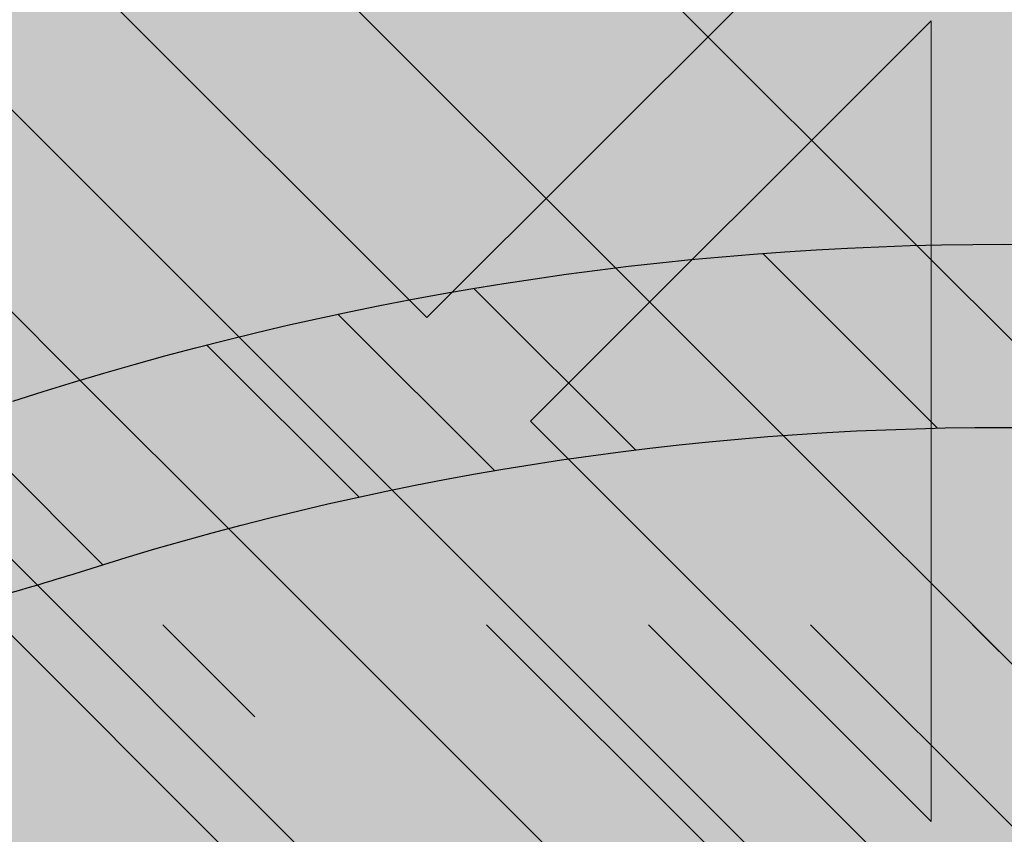
# Model space of a CAD drawing. Units: inches. Extents: x 844 to 2234, y 346 to 1084.
# Tile 80 of 93: x 2002.145 to 2003.858, y 707.323 to 708.742. Entities that reach past the tile are written whole.
import ezdxf

# ---------------------------------------------------------------- set-up
doc = ezdxf.new("R2010")
doc.units = ezdxf.units.IN
doc.header["$MEASUREMENT"] = 0
for name, color, linetype, lineweight in [('A-ANNO-DIMS', 2, 'Continuous', 18), ('furniture', 8, 'Continuous', 18), ('RA-AP-01$0$INT', 35, 'Continuous', 5)]:
    doc.layers.add(name, color=color, linetype=linetype, lineweight=lineweight)
doc.layers.add('RA-AP-01$0$FURN', color=3, linetype='Continuous')
doc.layers.add('RA-AP-01$0$WOOD', color=64, linetype='Continuous')
doc.styles.get("Standard").update_dxf_attribs({"font": 'arial.ttf'})
doc.dimstyles.get("Standard").update_dxf_attribs({"dimtxt": 6, "dimasz": 3, "dimexe": 0.18, "dimexo": 0.0625, "dimgap": 0.09, "dimtad": 0, "dimtih": 1, "dimtoh": 1, "dimdec": 1, "dimzin": 0, "dimdsep": 46, "dimlunit": 3, "dimtxsty": 'Standard', "dimblk": 'ARCHTICK', "dimcen": 0.09, "dimadec": 0, "dimazin": 0, "dimtfac": 1, "dimtdec": 1, "dimtofl": 0, "dimtmove": 0, "dimatfit": 3, "dimfxl": 1, "dimtolj": 1, "dimtzin": 0, "dimarcsym": 0})

# ---------------------------------------------------------------- blocks, each defined once
blk = doc.blocks.new('A$C18D01794')
at = {"layer": 'RA-AP-01$0$INT'}
h = blk.add_hatch(color=256, dxfattribs=at)
h.paths.add_polyline_path([(4.585917135068448, -7.856712009587804), (4.614201406330596, -7.856712009587056), (4.668846067270487, -7.802067348644738), (4.723490728212344, -7.856712009584164), (4.771774999457151, -7.856712009582887), (4.826419660396886, -7.80206734864072), (4.862780050090322, -7.838427738332541), (4.844495778842715, -7.856712009580965), (4.862780050090411, -7.856712009580482), (4.905206456960182, -7.814285602707865), (4.947632863832445, -7.856712009578238), (4.965917135079675, -7.856712009577755), (4.947632863831759, -7.838427738330656), (4.983993253523576, -7.802067348637219), (5.038637914464627, -7.856712009575829), (5.08692218571208, -7.856712009574554), (5.141566846649976, -7.802067348634224), (5.196211507589851, -7.856712009571666), (5.224495778822615, -7.856712009570916), (4.905206456953975, -7.537422687702283)])
h.paths.add_polyline_path([(4.895206456956031, -7.575706958950402), (4.895206456958921, -7.684996280828174), (4.840561796018589, -7.630351619890275)], flags=16)
h.paths.add_polyline_path([(4.915206456955638, -7.575706958949956), (4.969851117895509, -7.630351619887399), (4.915206456957609, -7.684996280827732)], flags=16)
h.paths.add_polyline_path([(4.826419660395175, -7.644493755514321), (4.881064321335613, -7.699138416452331), (4.771774999456703, -7.69913841645522)], flags=16)
h.paths.add_polyline_path([(4.983993253519558, -7.644493755510815), (5.038637914460456, -7.699138416449285), (4.929348592581548, -7.69913841645126)], flags=16)
h.paths.add_polyline_path([(4.881064321336025, -7.719138416452334), (4.826419660397532, -7.773783077393256), (4.771774999457062, -7.719138416455217)], flags=16)
h.paths.add_polyline_path([(4.929348592582019, -7.71913841645126), (5.038637914460982, -7.719138416449284), (4.983993253522945, -7.773783077389749)], flags=16)
h.paths.add_polyline_path([(4.895206456960191, -7.733280552075633), (4.895206456962115, -7.806001331460164), (4.876922185715016, -7.824285602708492), (4.840561796021581, -7.787925213016675)], flags=16)
h.paths.add_polyline_path([(4.915206456958487, -7.733280552075187), (4.969851117899527, -7.787925213013798), (4.933490728206909, -7.824285602708034), (4.9152064569598, -7.806001331461736)], flags=16)
h.paths.add_polyline_path([(4.757632863832376, -7.733280552079264), (4.812277524772842, -7.787925213017304), (4.757632863834348, -7.842569873958233)], flags=16)
h.paths.add_polyline_path([(4.737632863832376, -7.73328055207979), (4.737632863834348, -7.842569873958701), (4.682988202893906, -7.787925213020692)], flags=16)
h.paths.add_polyline_path([(5.05278005008503, -7.733280552072701), (5.052780050087917, -7.842569873951664), (4.998135389146995, -7.787925213013169)], flags=16)
h.paths.add_polyline_path([(5.072780050085024, -7.733280552072333), (5.127424711025931, -7.787925213010806), (5.072780050087916, -7.842569873951244)], flags=16)
h.paths.add_polyline_path([(4.935917135072783, -7.506712009583784), (5.255206456948811, -7.826001331459767), (5.255206456948932, -7.797717060211899), (5.200561796010279, -7.743072399273238), (5.255206456949403, -7.688427738334128), (5.25520645694961, -7.640143467086677), (5.200561796009787, -7.585498806146837), (5.236922185702417, -7.549138416454212), (5.255206456949919, -7.56742268770172), (5.255206456949998, -7.549138416454178), (5.212780050078687, -7.506712009583814), (5.25520645695036, -7.464285602712145), (5.255206456950438, -7.446001331464763), (5.236922185702424, -7.464285602712779), (5.200561796009796, -7.427925213020149), (5.255206456950753, -7.373280552079203), (5.25520645695096, -7.324996280834394), (5.200561796010322, -7.270351619893748), (5.255206456951428, -7.215706958952649), (5.255206456951547, -7.187422687705071)])
h.paths.add_polyline_path([(5.042988202883395, -7.42792521302065), (5.097632863823085, -7.373280552080975), (5.097632863822622, -7.482569873959883)], flags=16)
h.paths.add_polyline_path([(5.028846067259663, -7.442067348644384), (5.083490728198774, -7.496712009583504), (4.974201406321001, -7.496712009583035)], flags=16)
h.paths.add_polyline_path([(5.117632863823087, -7.37328055208089), (5.172277524762331, -7.42792521302015), (5.11763286382262, -7.482569873959851)], flags=16)
h.paths.add_polyline_path([(5.08349072819877, -7.516712009582191), (5.028846067259652, -7.571356670521302), (4.974201406320998, -7.516712009582638)], flags=16)
h.paths.add_polyline_path([(5.131774999446817, -7.35913841645716), (5.186419660386065, -7.413783077396415), (5.241064321325782, -7.359138416456712)], flags=17)
h.paths.add_polyline_path([(5.131774999446228, -7.496712009583703), (5.186419660386065, -7.442067348643883), (5.222780050079488, -7.478427738337313), (5.204495778832781, -7.496712009584014)], flags=16)
h.paths.add_polyline_path([(5.097632863822613, -7.530854145205813), (5.097632863823061, -7.640143467084723), (5.042988202883383, -7.585498806145032)], flags=16)
h.paths.add_polyline_path([(5.131774999446899, -7.339138416457162), (5.241064321325809, -7.339138416456712), (5.186419660386591, -7.284493755517479)], flags=17)
h.paths.add_polyline_path([(5.131774999446226, -7.516712009581999), (5.204495778830767, -7.516712009581702), (5.22278005007868, -7.534996280829206), (5.186419660386049, -7.571356670521828)], flags=16)
h.paths.add_polyline_path([(5.11763286382262, -7.530854145205852), (5.17227752476232, -7.585498806145562), (5.117632863823064, -7.64014346708481)], flags=16)
h.paths.add_polyline_path([(5.186419660386069, -7.599640941770585), (5.241064321325754, -7.654285602710281), (5.131774999446791, -7.654285602709814)], flags=16)
h.paths.add_polyline_path([(5.131774999446872, -7.674285602709813), (5.24106432132578, -7.674285602710282), (5.186419660386554, -7.728930263649504)], flags=16)
h.paths.add_polyline_path([(5.255206456951811, -7.126001331467467), (5.255206456951895, -7.106712009588038), (4.555206456956052, -7.106712009588038), (4.555206456956136, -7.12600133146746), (4.905206456953973, -7.476001331465289)])
h.paths.add_polyline_path([(4.983993253513404, -7.368930263651977), (4.92934859257295, -7.314285602713969), (5.03863791445186, -7.314285602711063)], flags=16)
h.paths.add_polyline_path([(4.969851117889988, -7.383072399276016), (4.915206456952556, -7.437717060215906), (4.915206456949648, -7.328427738338133)], flags=16)
h.paths.add_polyline_path([(4.929348592572535, -7.294285602713971), (4.983993253511019, -7.239640941773039), (5.038637914451496, -7.294285602711065)], flags=16)
h.paths.add_polyline_path([(5.052780050074912, -7.280143467087016), (4.998135389134438, -7.225498806148989), (5.052780050072919, -7.170854145208052)], flags=16)
h.paths.add_polyline_path([(5.07278005007491, -7.280143467086489), (5.072780050072918, -7.170854145207579), (5.127424711013374, -7.225498806145578)], flags=16)
h.paths.add_polyline_path([(4.89520645695295, -7.437717060216355), (4.840561796013067, -7.383072399278919), (4.895206456950961, -7.328427738338582)], flags=16)
h.paths.add_polyline_path([(4.915206456948365, -7.280143467090674), (4.915206456946434, -7.207422687704125), (4.933490728192729, -7.18913841645701), (4.969851117886972, -7.225498806149623)], flags=16)
h.paths.add_polyline_path([(4.881064321327021, -7.314285602715054), (4.82641966038902, -7.368930263655506), (4.771774999448108, -7.314285602717047)], flags=16)
h.paths.add_polyline_path([(4.895206456950073, -7.280143467091125), (4.840561796009022, -7.225498806152518), (4.876922185700835, -7.18913841645908), (4.895206456948749, -7.207422687706589)], flags=16)
h.paths.add_polyline_path([(4.983993253510392, -7.211356670525576), (4.947632863816944, -7.174996280833758), (4.965917135064043, -7.156712009585847), (5.038637914448995, -7.156712009584522)], flags=16)
h.paths.add_polyline_path([(4.881064321326543, -7.294285602715056), (4.771774999447578, -7.294285602717046), (4.826419660385607, -7.239640941776569)], flags=16)
h.paths.add_polyline_path([(4.905206456946447, -7.19913841645844), (4.862780050074785, -7.156712009587725), (4.947632863816685, -7.156712009586302)], flags=16)
h.paths.add_polyline_path([(5.14156684663679, -7.211356670521528), (5.086922185696452, -7.156712009583639), (5.196211507574223, -7.156712009581651)], flags=16)
h.paths.add_polyline_path([(4.8264196603837, -7.211356670529104), (4.771774999442643, -7.156712009590501), (4.8444957788276, -7.156712009588568), (4.862780050075511, -7.17499628083566)], flags=16)
h.paths.add_polyline_path([(4.812277524760289, -7.225498806153156), (4.757632863822258, -7.28014346709363), (4.757632863819352, -7.170854145214669)], flags=16)
h.paths.add_polyline_path([(4.73763286382226, -7.280143467093997), (4.682988202881349, -7.22549880615554), (4.737632863819352, -7.170854145215086)], flags=16)
h.paths.add_polyline_path([(4.723490728195188, -7.156712009591787), (4.668846067257299, -7.211356670532127), (4.614201406317417, -7.156712009594693)], flags=16)
h.paths.add_polyline_path([(4.597632863829262, -7.506712009583814), (4.555206456957951, -7.54913841645418), (4.555206456958029, -7.56742268770172), (4.573490728205535, -7.549138416454212), (4.609851117898167, -7.585498806146839), (4.555206456958338, -7.640143467086675), (4.555206456958546, -7.688427738334125), (4.60985111789767, -7.743072399273238), (4.555206456959015, -7.797717060211899), (4.555206456959138, -7.826001331459767), (4.874495778835167, -7.506712009583786), (4.5552064569564, -7.187422687705062), (4.555206456956523, -7.215706958952644), (4.609851117897629, -7.270351619893746), (4.555206456956988, -7.324996280834396), (4.555206456957198, -7.373280552079195), (4.609851117898153, -7.427925213020147), (4.573490728205528, -7.464285602712779), (4.555206456957507, -7.446001331464756), (4.555206456957585, -7.464285602712143)])
h.paths.add_polyline_path([(4.712780050085332, -7.482569873959882), (4.712780050084863, -7.373280552080972), (4.767424711024555, -7.42792521302065)], flags=16)
h.paths.add_polyline_path([(4.726922185709173, -7.496712009583504), (4.781566846648288, -7.442067348644384), (4.836211507586949, -7.496712009583033)], flags=16)
h.paths.add_polyline_path([(4.692780050085327, -7.482569873959851), (4.638135389145619, -7.427925213020149), (4.692780050084865, -7.373280552080892)], flags=16)
h.paths.add_polyline_path([(4.726922185709182, -7.516712009582191), (4.836211507586949, -7.51671200958264), (4.7815668466483, -7.571356670521304)], flags=16)
h.paths.add_polyline_path([(4.678637914461726, -7.496712009583706), (4.605917135075169, -7.496712009584014), (4.587632863828464, -7.478427738337311), (4.623993253521887, -7.442067348643881)], flags=16)
h.paths.add_polyline_path([(4.712780050085336, -7.530854145205816), (4.767424711024568, -7.585498806145034), (4.71278005008489, -7.640143467084724)], flags=16)
h.paths.add_polyline_path([(4.678637914461726, -7.516712009582001), (4.623993253521899, -7.571356670521829), (4.587632863829271, -7.534996280829206), (4.605917135077185, -7.5167120095817)], flags=16)
h.paths.add_polyline_path([(4.692780050085336, -7.530854145205848), (4.692780050084889, -7.64014346708481), (4.638135389145632, -7.585498806145562)], flags=16)
h.paths.add_polyline_path([(4.623993253521885, -7.413783077396415), (4.678637914461131, -7.359138416457161), (4.56934859258217, -7.359138416456712)], flags=17)
h.paths.add_polyline_path([(4.623993253521901, -7.599640941770568), (4.678637914461158, -7.654285602709814), (4.569348592582195, -7.654285602710281)], flags=16)
h.paths.add_polyline_path([(4.678637914461051, -7.339138416457162), (4.623993253521361, -7.284493755517479), (4.569348592582143, -7.339138416456712)], flags=17)
h.paths.add_polyline_path([(4.678637914461076, -7.674285602709813), (4.623993253521399, -7.728930263649504), (4.569348592582167, -7.674285602710281)], flags=16)
h = blk.add_hatch(color=256, dxfattribs=at)
h.paths.add_polyline_path([(4.905206456954232, -7.537422687702028), (4.874495778835232, -7.506712009583718), (4.555206456959138, -7.826001331459766), (4.555206456959269, -7.856712009588616), (4.585917135068449, -7.856712009587804)])
h.paths.add_polyline_path([(4.935917135072152, -7.506712009583152), (4.905206456953497, -7.537422687701806), (5.224495778822614, -7.856712009570917), (5.255206456948681, -7.856712009570104), (5.255206456948813, -7.826001331459768)])
h.paths.add_polyline_path([(5.255206456951549, -7.18742268770507), (5.255206456951813, -7.126001331467461), (4.905206456953563, -7.476001331465701), (4.935917135072559, -7.506712009584006)])
h.paths.add_polyline_path([(4.874495778835167, -7.506712009583785), (4.905206456953818, -7.476001331465132), (4.555206456956135, -7.126001331467458), (4.555206456956399, -7.187422687705064)])
h = blk.add_hatch(color=256, dxfattribs=at)
h.paths.add_polyline_path([(4.969851117891331, -7.630351619889621), (4.915206456952669, -7.575706958950966), (4.915206456952222, -7.684996280828739)])
h.paths.add_polyline_path([(4.895206456953064, -7.575706958950968), (4.840561796014413, -7.630351619889628), (4.895206456953533, -7.684996280828741)])
h.paths.add_polyline_path([(4.826419660390684, -7.644493755513362), (4.771774999451003, -7.699138416453052), (4.881064321329913, -7.699138416452587)])
h.paths.add_polyline_path([(4.881064321329884, -7.719138416452585), (4.771774999450921, -7.719138416453052), (4.82641966039018, -7.773783077392298)])
h.paths.add_polyline_path([(4.895206456953734, -7.733280552076196), (4.840561796013912, -7.787925213016031), (4.876922185707337, -7.824285602709455), (4.895206456954043, -7.806001331462747)])
h.paths.add_polyline_path([(4.862780050082808, -7.838427738332388), (4.826419660390178, -7.802067348639763), (4.771774999450351, -7.856712009579595), (4.844495778835303, -7.856712009579895)])
h.paths.add_polyline_path([(4.812277524766446, -7.787925213016036), (4.757632863827191, -7.733280552076788), (4.757632863826741, -7.842569873955747)])
h.paths.add_polyline_path([(4.737632863827191, -7.733280552076863), (4.682988202887508, -7.787925213016558), (4.737632863826743, -7.842569873955778)])
h.paths.add_polyline_path([(4.668846067263777, -7.802067348640287), (4.614201406325123, -7.856712009578949), (4.723490728202894, -7.856712009579402)])
h.paths.add_polyline_path([(4.905206456953846, -7.814285602708654), (4.862780050082654, -7.856712009579847), (4.947632863824561, -7.85671200958032)])
h.paths.add_polyline_path([(4.915206456952028, -7.733280552076195), (4.91520645695173, -7.806001331460731), (4.933490728199234, -7.824285602708648), (4.96985111789186, -7.787925213016022)])
h.paths.add_polyline_path([(5.038637914454841, -7.719138416453029), (4.929348592575874, -7.71913841645258), (4.983993253515593, -7.773783077392289)])
h.paths.add_polyline_path([(4.983993253515065, -7.644493755513352), (4.929348592575849, -7.699138416452582), (5.038637914454755, -7.699138416453031)])
h.paths.add_polyline_path([(5.052780050079843, -7.73328055207676), (4.998135389140595, -7.787925213016018), (5.052780050080309, -7.842569873955721)])
h.paths.add_polyline_path([(4.983993253516868, -7.802067348639752), (4.947632863824241, -7.838427738332383), (4.965917135071747, -7.856712009579888), (5.038637914456701, -7.856712009579572)])
h.paths.add_polyline_path([(5.127424711019533, -7.787925213016519), (5.072780050079843, -7.733280552076838), (5.07278005008031, -7.842569873955751)])
h.paths.add_polyline_path([(5.141566846643269, -7.802067348640248), (5.086922185704154, -7.85671200957937), (5.196211507581929, -7.856712009578901)])
for p, q in [((4.935917135072783, -7.506712009583784), (5.255206456948813, -7.826001331459769)), ((4.905206456953975, -7.537422687702283), (5.224495778822613, -7.856712009570916)), ((4.915206456955636, -7.575706958949957), (4.969851117895507, -7.630351619887399)), ((4.915206456957609, -7.684996280827729), (4.915206456955636, -7.575706958949957)), ((4.915206456957613, -7.684996280827727), (4.969851117895507, -7.630351619887399)), ((4.929348592581546, -7.69913841645126), (4.983993253519556, -7.644493755510815)), ((4.983993253519558, -7.644493755510817), (5.038637914460456, -7.699138416449285))]:
    blk.add_line(p, q, dxfattribs=at)
blk = doc.blocks.new('A$C32926AE1')
at = {"layer": 'RA-AP-01$0$FURN'}
h = blk.add_hatch(dxfattribs=at)
h.set_pattern_fill('ANSI31', color=256, scale=0.1, style=0)
h.set_pattern_definition([(45, (0, 0), (-0.0088388347648318, 0.0088388347648318), [])])
edge = h.paths.add_edge_path(flags=16)
edge.add_arc((4.904771284329206, 4.246793130718756), 0.2603971832811541, 75.22398030683196, 104.7760196931204)
edge.add_arc((4.904771284329206, 4.246793130718756), 0.2603971832811541, 75.223980306832, 104.77601969312039, ccw=False)
edge = h.paths.add_edge_path(flags=16)
edge.add_arc((4.904771284329206, 4.067062675376612), 0.2603971832811541, 255.2239803068796, 284.776019693168)
edge.add_arc((4.904771284329206, 4.067062675376612), 0.2603971832811541, 255.22398030687958, 284.77601969316805, ccw=False)
edge = h.paths.add_edge_path(flags=0)
edge.add_arc((4.904771284329206, 4.067062675376612), 0.2603971832811541, 255.2239803068796, 284.776019693168)
edge.add_arc((4.904771284329206, 4.067062675376612), 0.2603971832811541, 255.22398030687958, 284.77601969316805, ccw=False)
edge = h.paths.add_edge_path(flags=0)
edge.add_arc((4.904771284329206, 4.067062675376612), 0.2603971832811541, 255.2239803068796, 284.776019693168)
edge.add_arc((4.904771284329206, 4.067062675376612), 0.2603971832811541, 255.22398030687958, 284.77601969316805, ccw=False)
edge = h.paths.add_edge_path()
edge.add_arc((4.604388392048174, 4.588829985554312), 0.1599999999999918, 342.3781640246255, 354.4317409793762)
edge.add_arc((5.090145208887507, 4.43216705527679), 0.3503971832811637, 162.0091218307731, 180.3186872093483)
edge.add_arc((5.205154176610243, 4.588829985554953), 0.1599999999999917, 185.5682590208461, 197.6218359767349)
edge.add_arc((4.904771284329229, 4.246793130718735), 0.3503971832811761, 72.00912183053516, 107.9908781690354)
edge.add_arc((9.535952835716557, 4.28682295566602), 4.798342501046485, 178.2875002453811, 181.5576802719453)
edge.add_arc((4.719397359771122, 4.43216705527679), 0.3503971832811637, 359.6813127906516, 377.9908781692269)
edge.add_arc((9.535967292294904, 4.286822350292874), 4.778371420254705, 178.2965938931842, 181.5667745797229)
edge.add_arc((4.719397359771122, 4.43216705527679), 0.3303971832811637, 359.6813127906516, 377.9908781692269)
edge.add_arc((0.2735752763637294, 4.286822350292874), 4.7783714202547, 358.4332254202771, 361.7034061068158)
edge.add_arc((5.061434214606998, 4.732549947558029), 0.1600000000000254, 252.3781640250584, 264.4317409792362)
edge.add_arc((4.748108354051257, 4.732549947558012), 0.1600000000000541, 275.5682590208426, 287.6218359759532)
edge.add_arc((4.604388392048115, 4.588829985554317), 0.1800000000000505, 342.3567572500182, 349.3735009646207)
edge.add_arc((5.205154176610254, 4.588829985554976), 0.1800000000000069, 190.6264990356027, 197.6432427513933)
edge.add_arc((5.061434214607106, 4.732549947558013), 0.1800000000000424, 252.3567572496606, 259.3735009644582)
edge.add_arc((4.904771284329208, 4.246793130718737), 0.3303971832811676, 71.99844483668534, 108.0015551637021)
edge.add_arc((4.748108354051414, 4.732549947558045), 0.1800000000000547, 280.6264990355479, 287.6432427495938)
edge.add_arc((5.090145208887514, 4.432167055276789), 0.2803971832811691, 162.8706300666893, 180.816523289902)
edge.add_arc((4.719397359771136, 4.432167055276689), 0.2803971832811534, 359.183476710103, 377.1293699333214)
edge.add_arc((4.904771284329222, 4.246793130718737), 0.2803971832811769, 72.87063006672916, 107.1293699332334)
edge.add_arc((5.090145208887522, 4.432167055276788), 0.2603971832811776, 165.2239803068007, 180.9953123810312)
edge.add_arc((4.719397359771141, 4.432167055276699), 0.2603971832811458, 359.0046876189768, 374.7760196932087)
edge.add_arc((5.090145208887507, 4.43216705527679), 0.3303971832811637, 162.0091218307731, 180.3186872093483)
edge.add_arc((9.53595427642584, 4.285015535491528), 4.728345371032053, 178.265043920078, 181.5679956281801)
edge.add_arc((0.2735882922327999, 4.285015535491582), 4.728345371032045, 358.4320043718193, 361.7349560799204)
edge.add_arc((9.535953591267507, 4.284458026472751), 4.708343996644348, 178.2573054306777, 181.5704995759608)
edge.add_arc((0.273588977391114, 4.284458026472785), 4.708343996644358, 358.4295004240388, 361.7426945693213)
edge.add_arc((0.2735889773911131, 4.029397779622582), 4.708343996644359, 358.2573054306787, 361.5704995759613)
edge.add_arc((9.535953591267518, 4.029397779622618), 4.708343996644359, 178.4295004240391, 181.7426945693223)
edge.add_arc((0.2735882922327901, 4.028840270603786), 4.728345371032054, 358.2650439200796, 361.5679956281808)
edge.add_arc((9.53595427642584, 4.028840270603841), 4.728345371032054, 178.4320043718199, 181.7349560799219)
edge.add_arc((0.2735752763637302, 4.027033455802493), 4.778371420254699, 358.2965938931842, 361.5667745797229)
edge.add_arc((4.719397359771122, 3.881688750818578), 0.3303971832811637, 342.0091218307731, 360.3186872093484)
edge.add_arc((5.090145208887507, 3.881688750818578), 0.3303971832811637, 179.6813127906516, 197.9908781692269)
edge.add_arc((9.535967292294904, 4.027033455802493), 4.778371420254705, 178.433225420277, 181.7034061068158)
edge.add_arc((4.719397359771122, 3.881688750818578), 0.3503971832811637, 342.0091218307731, 360.3186872093484)
edge.add_arc((9.53595283571655, 4.027032850429349), 4.79834250104648, 178.4423197280546, 181.7124997546188)
edge.add_arc((4.719397359771141, 3.881688750818669), 0.2603971832811458, 345.2239803067913, 360.9953123810232)
edge.add_arc((5.090145208887522, 3.88168875081858), 0.2603971832811776, 179.0046876189687, 194.7760196931993)
edge.add_arc((4.904771284329222, 4.067062675376631), 0.2803971832811769, 252.8706300667665, 287.1293699332708)
edge.add_arc((4.719397359771136, 3.881688750818678), 0.2803971832811534, 342.8706300666787, 360.8165232898969)
edge.add_arc((5.090145208887514, 3.881688750818579), 0.2803971832811691, 179.183476710098, 197.1293699333106)
edge.add_arc((4.748108354051414, 3.581305858537323), 0.1800000000000547, 72.3567572504062, 79.37350096445199)
edge.add_arc((4.904771284329208, 4.067062675376631), 0.3303971832811676, 251.9984448362979, 288.0015551633146)
edge.add_arc((5.061434214607106, 3.581305858537355), 0.1800000000000424, 100.6264990355418, 107.6432427503394)
edge.add_arc((5.205154176610254, 3.725025820540392), 0.1800000000000069, 162.3567572486066, 169.3735009643972)
edge.add_arc((4.604388392048115, 3.725025820541051), 0.1800000000000505, 10.62649903537925, 17.64324274998182)
edge.add_arc((4.748108354051257, 3.581305858537356), 0.1600000000000541, 72.37816402404681, 84.43174097915735)
edge.add_arc((4.904771284329229, 4.067062675376632), 0.3503971832811761, 252.0091218309645, 287.9908781694648)
edge.add_arc((5.061434214606998, 3.581305858537339), 0.1600000000000254, 95.56825902076373, 107.6218359749416)
edge.add_arc((5.205154176610243, 3.725025820540414), 0.1599999999999917, 162.3781640232651, 174.4317409791539)
edge.add_arc((5.090145208887507, 3.881688750818578), 0.3503971832811637, 179.6813127906516, 197.9908781692269)
edge.add_arc((4.604388392048174, 3.725025820541056), 0.1599999999999918, 5.568259020623824, 17.62183597537444)
edge.add_arc((0.2735897329420762, 4.28682295566602), 4.798342501046482, 358.4423197280547, 361.7124997546188)
edge.add_arc((0.2735897329420691, 4.027032850429348), 4.798342501046489, 358.2875002453812, 361.5576802719453)
at = {"layer": 'RA-AP-01$0$WOOD'}
h = blk.add_hatch(color=256, dxfattribs=at)
h.dxf.hatch_style = 1
h.paths.add_polyline_path([(5.157430609644524, 4.573483066760929, -0.1009492694046607), (5.155401577623758, 4.593365984175333, -0.1842662638101597), (5.172249623284174, 4.638795604568598, 0.2056608120311276), (5.179560981299304, 4.661316324430096, 0.3614336704623542), (5.134352340494423, 4.706524965234944, 0.2056608120311297), (5.111831620632933, 4.699213607219793, -0.1842662638101113), (5.066402000239693, 4.682365561559342, -0.1055311479399994), (5.045656153913092, 4.68467289944697, 0.1567636581983829), (4.763886414745334, 4.684672899446966, -0.1055311479399895), (4.743140568418733, 4.68236556155934, -0.1842662638100833), (4.6977109480255, 4.69921360721979, 0.2056608120302612), (4.675190228164109, 4.706524965234949, 0.3614336704708441), (4.629981587358889, 4.66131632442871, 0.2056608120245944), (4.637292945374126, 4.638795604567974, -0.1842662638101024), (4.654140991034615, 4.59336598417475, -0.1009492694055169), (4.652111959013835, 4.573483066760181, 0.021410119221476), (4.629748025606143, 4.156712009541676, 0.0214101192214795), (4.652111959013809, 3.739940952323101, -0.1009492694059586), (4.654140991034615, 3.720058034908448, -0.1842662638100975), (4.637292945374126, 3.674628414515226, 0.2056608120245705), (4.629981587358889, 3.652107694654492, 0.3614336704708879), (4.675190228164113, 3.606899053848249, 0.2056608120302384), (4.697710948025501, 3.614210411863408, -0.1842662638100995), (4.743140568418738, 3.63105845752386, -0.1055311479402541), (4.763886414745388, 3.628751119636215, 0.1567636581983776), (5.045656153913137, 3.628751119636244, -0.1055311479397538), (5.066402000239692, 3.631058457523857, -0.1842662638101067), (5.111831620632931, 3.614210411863407, 0.2056608120310924), (5.134352340494417, 3.606899053848256, 0.3614336704624001), (5.179560981299307, 3.652107694653103, 0.2056608120311314), (5.172249623284175, 3.6746284145146, -0.1842662638101402), (5.155401577623758, 3.72005803490786, -0.1009492694051366), (5.15743060964455, 3.739940952322354, 0.0214101192215073), (5.179794543052287, 4.156712009541468, 0.0214101192215252)])
h.paths.add_polyline_path([(4.639748609479751, 4.156712009541513, 0.0213537860821624), (4.661970494867118, 3.741887061152232, -0.094075836301374), (4.664143710413708, 3.7196126951003, -0.1824818158568985), (4.644813765429836, 3.668037719127816, 0.2056608120245319), (4.639939526753007, 3.653023905887301, 0.3614336704710246), (4.676106439397173, 3.616856993242342, 0.2056608120302234), (4.691120252638095, 3.621731231919122, -0.1824818158602558), (4.742695228611606, 3.641061176902986, -0.1029891339458722), (4.766991894714349, 3.638256818950944, 0.156709409989566), (5.042550673941472, 3.638256818950105, -0.102989133958497), (5.066847340047078, 3.641061176902949, -0.1824818158594995), (5.118422316020358, 3.621731231919103, 0.2056608120311416), (5.133436129261316, 3.616856993242346, 0.3614336704621468), (5.169603041905217, 3.653023905886178, 0.2056608120310986), (5.164728803228477, 3.668037719127177, -0.1824818158565612), (5.145398858244737, 3.719612695099578, -0.0940758363009313), (5.147572073791232, 3.741887061151398, 0.0213537860822023), (5.169793959178681, 4.156712009541451, 0.0213537860822226), (5.147572073791203, 4.571536957931898, -0.0940758363005034), (5.145398858244737, 4.59381132398362, -0.1824818158565587), (5.164728803228476, 4.645386299956021, 0.2056608120311045), (5.169603041905216, 4.66040011319702, 0.3614336704621845), (5.133436129261313, 4.696567025840856, 0.2056608120310773), (5.118422316020359, 4.691692787164098, -0.182481815859508), (5.066847340047078, 4.67236284218025, -0.1029891339584606), (5.04255067394148, 4.675167200133092, 0.156709409989566), (4.766991894714357, 4.675167200132257, -0.1029891339458842), (4.742695228611611, 4.672362842180213, -0.1824818158602725), (4.691120252638095, 4.691692787164077, 0.2056608120302152), (4.676106439397174, 4.696567025840858, 0.3614336704710363), (4.639939526753005, 4.660400113195899, 0.2056608120245495), (4.644813765429837, 4.645386299955384, -0.1824818158568934), (4.664143710413708, 4.593811323982902, -0.0940758363009187), (4.661970494867149, 4.571536957931074, 0.021353786082177)], flags=16)
h.paths.add_polyline_path([(5.129794543052235, 4.432167055276933, -0.0141661062790638), (5.130152669293814, 4.156927903047693, -0.0141661062790647), (5.129794543052234, 3.881688750818433, -0.0785247771143638), (5.10979738006795, 3.755143611847103, 0.0945969212073497), (5.105408519571111, 3.717898134952927, 0.1043170707844957), (5.116074640131521, 3.670385395016088, 0.1043170707864965), (5.068561900193738, 3.681051515576561, 0.09459692119553), (5.031316423304057, 3.676662655080835, -0.1580239521427272), (4.778226145355827, 3.676662655080367, 0.0945969211986668), (4.740980668464973, 3.681051515576592, 0.1043170707882822), (4.693467928526415, 3.670385395015844, 0.1043170707867916), (4.704134049087309, 3.717898134953662, 0.0945969211972894), (4.69974518859162, 3.755143611844042, -0.0785247771163196), (4.679748025606343, 3.881688750818406, -0.0141661062790663), (4.679389899364763, 4.156927903047693, -0.0141661062790672), (4.679748025606343, 4.432167055276998, -0.0785247771163064), (4.699745188591625, 4.55871219425134, 0.094596921197333), (4.704134049087308, 4.595957671141738, 0.1043170707867205), (4.693467928526416, 4.643470411079523, 0.1043170707882628), (4.740980668464965, 4.632804290518776, 0.0945969211988114), (4.778226145355874, 4.637193151015016, -0.158023952142669), (5.031316423304015, 4.637193151014546, 0.0945969211956361), (5.068561900193736, 4.632804290518806, 0.1043170707864979), (5.11607464013152, 4.643470411079278, 0.1043170707844617), (5.105408519571112, 4.595957671142455, 0.0945969212074597), (5.109797380067959, 4.558712194248236, -0.0785247771143467)], flags=0)
h.paths.add_polyline_path([(5.119794532311105, 4.432259799204851, -0.0142000800617244), (5.120156169157484, 4.156927903047701, -0.0142000800617277), (5.119794532311105, 3.881596006890482, -0.0784894509520253), (5.100273383573699, 3.758192358677797, 0.0940138827242913), (5.095413455884425, 3.717477693979438, 0.0606271852308753), (5.099615656341024, 3.686844378806616, 0.0606271852322524), (5.068982341167493, 3.691046579263239, 0.0940138827010453), (5.028267676478798, 3.686186651576848, -0.1580706864508061), (4.781274892180912, 3.686186651576435, 0.0940138827026903), (4.740560227491556, 3.691046579263279, 0.0606271852339895), (4.709926912317155, 3.686844378806508, 0.0606271852329405), (4.714129112773991, 3.717477693980356, 0.094013882701304), (4.709269185087677, 3.758192358669163, -0.0784894509577193), (4.689748036347473, 3.881596006890469, -0.014200080061729), (4.689386399501094, 4.156927903047709, -0.0142000800617217), (4.689748036347473, 4.432259799204808, -0.078489450957724), (4.709269185087651, 4.555663447426125, 0.0940138827014585), (4.714129112773992, 4.596378112114996, 0.0606271852329731), (4.709926912317154, 4.62701142728886, 0.0606271852340196), (4.74056022749157, 4.622809226832087, 0.0940138827024997), (4.781274892180847, 4.627669154518912, -0.1580706864508359), (5.028267676478777, 4.627669154518526, 0.0940138827010946), (5.068982341167492, 4.622809226832129, 0.060627185232254), (5.099615656341024, 4.627011427288751, 0.0606271852308727), (5.095413455884425, 4.59637811211593, 0.0940138827241088), (5.100273383573675, 4.555663447417647, -0.0784894509520978)], flags=0)
h.paths.add_polyline_path([(5.06978912287499, 4.430218106756144, -0.014241683694547), (5.070173729147532, 4.156927903047672, -0.0142416836945458), (5.06978912287499, 3.883637699339223, -0.0800609523125196), (5.052662118612511, 3.773463122773442, 0.0526421978001116), (5.04590916754064, 3.740550867606997, 0.0526421977992423), (5.012996912374707, 3.73379791653534, -0.1583028414718258), (4.796545656286308, 3.73379791653451, 0.0526421978034211), (4.763633401117837, 3.740550867607021, 0.0526421978018622), (4.756880450045755, 3.773463122774558, -0.0800609523117106), (4.739753445783639, 3.883637699339268, -0.0142416836945435), (4.739368839511098, 4.156927903047671, -0.0142416836945477), (4.739753445783639, 4.430218106756155, -0.0800609523116345), (4.75688045004574, 4.540392683320762, 0.052642197801941), (4.763633401117837, 4.573304938488346, 0.0526421978035071), (4.796545656286361, 4.580057889560873, -0.1583028414717561), (5.012996912374669, 4.580057889560039, 0.0526421977993048), (5.04590916754064, 4.57330493848837, 0.0526421978002057), (5.052662118612529, 4.540392683321868, -0.080060952312477)], flags=0)
h.paths.add_polyline_path([(5.049789715110557, 4.43038092723357, -0.0143097550741839), (5.05018085590259, 4.156927903047715, -0.0143097550741854), (5.049789715110558, 3.883474878861827, -0.0800685599149176), (5.03362098255317, 3.779581877367999, 0.0306258898956367), (5.028241146483733, 3.758218888663947, 0.0306258898977031), (5.006878157778253, 3.75283905259408, -0.1583983521624096), (4.802664410878162, 3.752839052594731, 0.0306258898946014), (4.781301422174808, 3.758218888663924, 0.0306258898967912), (4.775921586105202, 3.779581877368794, -0.080068559914251), (4.759752853548071, 3.883474878861786, -0.0143097550741854), (4.759361712756037, 4.156927903047671, -0.0143097550741854), (4.759752853548071, 4.430380927233557, -0.0800685599142479), (4.775921586105193, 4.534273928726546, 0.0306258898968306), (4.781301422174808, 4.555636917431444, 0.0306258898945754), (4.802664410878143, 4.561016753500631, -0.1583983521624168), (5.006878157778244, 4.561016753501291, 0.0306258898977177), (5.028241146483733, 4.555636917431421, 0.0306258898958182), (5.03362098255321, 4.534273928727244, -0.080068559914796)], flags=0)
h.paths.add_polyline_path([(4.999766070382627, 4.428171244713864, -0.0143443147609634), (5.000198441819402, 4.156927903047689, -0.0143443147609612), (4.999766070382627, 3.885684561381556, -0.0784641635803329), (4.987356730658798, 3.799103304488872, -0.1506053783831347), (4.822185837999821, 3.79910330448882, -0.0784641635803318), (4.809776498276007, 3.885684561381509, -0.014344314760963), (4.809344126839227, 4.156927903047677, -0.0143443147609645), (4.809776498276007, 4.428171244713873, -0.0784641635803192), (4.822185837999822, 4.514752501606549, -0.1506053783831338), (4.987356730658798, 4.514752501606494, -0.078464163580285)], flags=0)
h.paths.add_polyline_path([(4.979755254238824, 4.42764379880488, -0.0143772539198268), (4.980205517789977, 4.156927903047693, -0.0143772539198275), (4.979755254238824, 3.886212007290489, -0.0689242507424422), (4.971183264704897, 3.815276770442801, -0.1296645318904179), (4.838359303953726, 3.815276770442746, -0.0689242507424186), (4.829787314419809, 3.886212007290419, -0.0143772539198292), (4.829337050868653, 4.156927903047653, -0.0143772539198325), (4.829787314419809, 4.427643798804946, -0.0689242507424211), (4.838359303953725, 4.498579035652621, -0.1296645318904187), (4.971183264704897, 4.498579035652565, -0.0689242507424401)], flags=0)
h = blk.add_hatch(color=256, dxfattribs=at)
h.dxf.hatch_style = 1
h.paths.add_polyline_path([(5.145398858244737, 4.59381132398362, -0.1824818158565616), (5.164728803228476, 4.645386299956021, 0.2056608120311045), (5.169603041905216, 4.66040011319702, 0.3614336704621845), (5.133436129261313, 4.696567025840856, 0.2056608120310773), (5.118422316020359, 4.691692787164098, -0.182481815859508), (5.066847340047078, 4.67236284218025, -0.1029891339584606), (5.04255067394148, 4.675167200133092, 0.156709409989566), (4.766991894714357, 4.675167200132257, -0.1029891339458842), (4.742695228611611, 4.672362842180213, -0.1824818158602725), (4.691120252638095, 4.691692787164077, 0.2056608120302152), (4.676106439397174, 4.696567025840858, 0.3614336704710363), (4.639939526753005, 4.660400113195899, 0.2056608120245495), (4.644813765429837, 4.645386299955384, -0.1824818158568934), (4.664143710413708, 4.593811323982902, -0.0940758363009187), (4.661970494867149, 4.571536957931074, 0.0213537860821772), (4.639748609479751, 4.156712009541507, 0.0213537860821625), (4.661970494867119, 3.741887061152226, -0.0940758363013071), (4.664143710413708, 3.719612695100309, -0.1824818158569294), (4.644813765429836, 3.668037719127816, 0.2056608120245319), (4.639939526753007, 3.653023905887301, 0.3614336704710246), (4.676106439397173, 3.616856993242342, 0.2056608120302234), (4.691120252638095, 3.621731231919122, -0.1824818158602558), (4.742695228611606, 3.641061176902986, -0.1029891339458722), (4.766991894714349, 3.638256818950944, 0.156709409989566), (5.042550673941472, 3.638256818950105, -0.102989133958497), (5.066847340047078, 3.641061176902949, -0.1824818158594995), (5.118422316020358, 3.621731231919103, 0.2056608120311416), (5.133436129261316, 3.616856993242346, 0.3614336704621468), (5.169603041905217, 3.653023905886178, 0.2056608120310986), (5.164728803228477, 3.668037719127177, -0.1824818158565612), (5.145398858244737, 3.719612695099578, -0.0940758363009313), (5.147572073791232, 3.741887061151398, 0.0213537860822023), (5.169793959178681, 4.156712009541451, 0.0213537860822226), (5.147572073791203, 4.571536957931898, -0.0940758363004996)])
h.paths.add_polyline_path([(5.109797380067958, 4.55871219424824, -0.0785247771143472), (5.129794543052234, 4.432167055276936, -0.0141661062790644), (5.130152669293814, 4.156927903047685, -0.014166106279066), (5.129794543052234, 3.881688750818401, -0.0785247771143517), (5.109797380067946, 3.755143611847092, 0.0945969212073132), (5.105408519571111, 3.717898134952929, 0.1043170707844995), (5.116074640131521, 3.670385395016088, 0.1043170707864965), (5.068561900193738, 3.681051515576561, 0.09459692119553), (5.031316423304057, 3.676662655080835, -0.1580239521427272), (4.778226145355827, 3.676662655080367, 0.0945969211986668), (4.740980668464973, 3.681051515576592, 0.1043170707882822), (4.693467928526415, 3.670385395015844, 0.1043170707867916), (4.704134049087309, 3.717898134953662, 0.0945969211972894), (4.69974518859162, 3.755143611844042, -0.0785247771163196), (4.679748025606343, 3.881688750818406, -0.0141661062790663), (4.679389899364763, 4.156927903047693, -0.0141661062790672), (4.679748025606343, 4.432167055276998, -0.0785247771163064), (4.699745188591625, 4.55871219425134, 0.094596921197333), (4.704134049087308, 4.595957671141738, 0.1043170707867205), (4.693467928526416, 4.643470411079523, 0.1043170707882628), (4.740980668464965, 4.632804290518776, 0.0945969211988114), (4.778226145355874, 4.637193151015016, -0.158023952142669), (5.031316423304015, 4.637193151014546, 0.0945969211956361), (5.068561900193736, 4.632804290518806, 0.1043170707864979), (5.11607464013152, 4.643470411079278, 0.1043170707844617), (5.105408519571112, 4.595957671142455, 0.0945969212074504)], flags=16)
h.paths.add_polyline_path([(5.100273383573655, 4.55566344741771, -0.0784894509521388), (5.119794532311105, 4.432259799204852, -0.0142000800617252), (5.120156169157484, 4.156927903047686, -0.014200080061726), (5.119794532311105, 3.881596006890502, -0.0784894509520446), (5.100273383573696, 3.758192358677786, 0.0940138827242721), (5.095413455884425, 3.717477693979436, 0.0606271852308692), (5.099615656341024, 3.686844378806616, 0.0606271852322522), (5.068982341167493, 3.691046579263239, 0.0940138827010453), (5.028267676478798, 3.686186651576848, -0.1580706864508061), (4.781274892180912, 3.686186651576435, 0.0940138827026903), (4.740560227491556, 3.691046579263279, 0.0606271852339895), (4.709926912317155, 3.686844378806508, 0.0606271852329405), (4.714129112773991, 3.717477693980356, 0.094013882701304), (4.709269185087677, 3.758192358669163, -0.0784894509577193), (4.689748036347473, 3.881596006890469, -0.014200080061729), (4.689386399501094, 4.156927903047709, -0.0142000800617217), (4.689748036347473, 4.432259799204808, -0.078489450957724), (4.709269185087651, 4.555663447426125, 0.0940138827014585), (4.714129112773992, 4.596378112114996, 0.0606271852329731), (4.709926912317154, 4.62701142728886, 0.0606271852340196), (4.74056022749157, 4.622809226832087, 0.0940138827024997), (4.781274892180847, 4.627669154518912, -0.1580706864508359), (5.028267676478777, 4.627669154518526, 0.0940138827010946), (5.068982341167492, 4.622809226832129, 0.060627185232254), (5.099615656341024, 4.627011427288751, 0.0606271852308727), (5.095413455884425, 4.59637811211593, 0.094013882723957)], flags=0)
h.paths.add_polyline_path([(5.04590916754064, 4.57330493848837, 0.0526421978002057), (5.052662118612529, 4.540392683321868, -0.0800609523124783), (5.06978912287499, 4.430218106756142, -0.0142416836945469), (5.070173729147532, 4.156927903047672, -0.0142416836945458), (5.06978912287499, 3.883637699339223, -0.0800609523125196), (5.052662118612511, 3.773463122773442, 0.0526421978001116), (5.04590916754064, 3.740550867606997, 0.0526421977992423), (5.012996912374707, 3.73379791653534, -0.1583028414718258), (4.796545656286308, 3.73379791653451, 0.0526421978034211), (4.763633401117837, 3.740550867607021, 0.0526421978018622), (4.756880450045755, 3.773463122774558, -0.0800609523117106), (4.739753445783639, 3.883637699339268, -0.0142416836945435), (4.739368839511098, 4.156927903047671, -0.0142416836945477), (4.739753445783639, 4.430218106756155, -0.0800609523116345), (4.75688045004574, 4.540392683320762, 0.052642197801941), (4.763633401117837, 4.573304938488346, 0.0526421978035071), (4.796545656286361, 4.580057889560873, -0.1583028414717561), (5.012996912374669, 4.580057889560039, 0.0526421977993048)], flags=0)
h.paths.add_polyline_path([(5.028241146483733, 4.555636917431422, 0.0306258898956949), (5.033620982553182, 4.534273928727329, -0.0800685599148649), (5.049789715110557, 4.430380927233569, -0.0143097550741839), (5.05018085590259, 4.156927903047715, -0.0143097550741854), (5.049789715110558, 3.883474878861827, -0.0800685599149176), (5.03362098255317, 3.779581877367999, 0.0306258898956367), (5.028241146483733, 3.758218888663947, 0.0306258898977031), (5.006878157778253, 3.75283905259408, -0.1583983521624096), (4.802664410878162, 3.752839052594731, 0.0306258898946014), (4.781301422174808, 3.758218888663924, 0.0306258898967912), (4.775921586105202, 3.779581877368794, -0.080068559914251), (4.759752853548071, 3.883474878861786, -0.0143097550741854), (4.759361712756037, 4.156927903047671, -0.0143097550741854), (4.759752853548071, 4.430380927233557, -0.0800685599142479), (4.775921586105193, 4.534273928726546, 0.0306258898968306), (4.781301422174808, 4.555636917431444, 0.0306258898945754), (4.802664410878143, 4.561016753500631, -0.1583983521624168), (5.006878157778244, 4.561016753501291, 0.0306258898977174)], flags=0)
h.paths.add_polyline_path([(4.987356730658798, 4.514752501606494, -0.0784641635803018), (4.999766070382627, 4.428171244713845, -0.0143443147609637), (5.000198441819402, 4.156927903047665, -0.0143443147609622), (4.999766070382628, 3.885684561381514, -0.0784641635802952), (4.987356730658797, 3.799103304488872, -0.1506053783831338), (4.822185837999821, 3.799103304488819, -0.0784641635803342), (4.809776498276007, 3.885684561381512, -0.0143443147609628), (4.809344126839227, 4.156927903047676, -0.0143443147609646), (4.809776498276007, 4.428171244713873, -0.0784641635803192), (4.822185837999822, 4.514752501606549, -0.1506053783831338)], flags=0)
h.paths.add_polyline_path([(4.971183264704897, 4.498579035652566, -0.0689242507424384), (4.979755254238824, 4.427643798804883, -0.0143772539198276), (4.980205517789977, 4.15692790304768, -0.0143772539198258), (4.979755254238823, 3.88621200729051, -0.0689242507424628), (4.971183264704897, 3.815276770442801, -0.129664531890417), (4.838359303953726, 3.815276770442746, -0.0689242507424186), (4.829787314419809, 3.886212007290419, -0.0143772539198292), (4.829337050868653, 4.156927903047653, -0.0143772539198325), (4.829787314419809, 4.427643798804946, -0.0689242507424211), (4.838359303953725, 4.498579035652621, -0.1296645318904187)], flags=0)
h = blk.add_hatch(dxfattribs=at)
h.set_pattern_fill('ANSI31', color=256, scale=0.05, style=0)
h.set_pattern_definition([(45, (0, 0), (-0.0044194173824159, 0.0044194173824159), [])])
h.paths.add_polyline_path([(5.130152669293814, 4.156927903047704, 0.0141661062790657), (5.129794543052234, 4.432167055276982, 0.0777827904001433), (5.110168979996553, 4.557559993161921, -0.0976515123401879), (5.105408519571111, 4.595957671142454, -0.1043170707844687), (5.116074640131522, 4.64347041107928), (5.099615656341024, 4.627011427288751, 0.0606271852308727), (5.095413455884425, 4.59637811211593, 0.0940138827241088), (5.100273383573675, 4.555663447417647, -0.0784894509520972), (5.119794532311105, 4.432259799204852, -0.0142000800617252), (5.120156169157484, 4.156927903047686, -0.014200080061726), (5.119794532311105, 3.881596006890502, -0.0784894509520446), (5.100273383573696, 3.758192358677786, 0.0940138827242721), (5.095413455884425, 3.717477693979436, 0.0606271852308692), (5.099615656341024, 3.686844378806616), (5.116074640131519, 3.67038539501609, -0.1043170707844594), (5.105408519571112, 3.717898134952912, -0.0976515123401594), (5.11016897999655, 3.756295812933435, 0.0777827904001654), (5.129794543052234, 3.881688750818409, 0.0141661062790665)])
h.paths.add_polyline_path([(5.030164222210597, 3.676291055149937, -0.0976515123472002), (5.068561900193739, 3.681051515576561, -0.1043170707864927), (5.116074640131521, 3.670385395016088), (5.099615656341024, 3.686844378806616, 0.0606271852322522), (5.068982341167493, 3.691046579263239, 0.0940138827010453), (5.028267676478798, 3.686186651576848, -0.1580706864508061), (4.781274892180912, 3.686186651576435, 0.0940138827026903), (4.740560227491556, 3.691046579263279, 0.0606271852339913), (4.709926912317154, 3.686844378806508), (4.693467928526416, 3.670385395015845, -0.1043170707882796), (4.740980668464973, 3.681051515576592, -0.0976515123427246), (4.779378346446416, 3.676291055150394, 0.156512506893803)])
h.paths.add_polyline_path([(4.689748036347473, 3.881596006890472, -0.014200080061729), (4.689386399501094, 4.156927903047712, -0.0142000800617195), (4.689748036347473, 4.432259799204768, -0.078489450957742), (4.709269185087648, 4.555663447426114, 0.0940138827014821), (4.714129112773992, 4.596378112114995, 0.0606271852329748), (4.709926912317154, 4.62701142728886), (4.693467928526414, 4.643470411079524, -0.1043170707867939), (4.704134049087309, 4.595957671141706, -0.09765151234893), (4.699373588660725, 4.557559993157876, 0.0777827903975372), (4.679748025606343, 4.432167055276987, 0.0141661062790675), (4.679389899364763, 4.156927903047675, 0.0141661062790641), (4.679748025606343, 3.88168875081843, 0.0777827903975637), (4.699373588660724, 3.756295812937497, -0.0976515123490278), (4.704134049087308, 3.717898134953629, -0.1043170707867196), (4.693467928526416, 3.670385395015845), (4.709926912317155, 3.686844378806508, 0.0606271852329413), (4.714129112773991, 3.717477693980357, 0.0940138827013084), (4.709269185087676, 3.758192358669166, -0.0784894509577192)])
h.paths.add_polyline_path([(4.779378346446434, 4.63756475094498, -0.0976515123427943), (4.740980668464964, 4.632804290518776, -0.1043170707882609), (4.693467928526416, 4.643470411079523), (4.709926912317154, 4.62701142728886, 0.0606271852340196), (4.74056022749157, 4.622809226832087, 0.0940138827024997), (4.781274892180847, 4.627669154518912, -0.1580706864508359), (5.028267676478777, 4.627669154518526, 0.0940138827010946), (5.068982341167492, 4.622809226832129, 0.060627185232254), (5.099615656341024, 4.627011427288751), (5.116074640131521, 4.643470411079279, -0.1043170707865022), (5.068561900193735, 4.632804290518806, -0.0976515123475899), (5.030164222210446, 4.637564750945479, 0.1565125068936924)])
h = blk.add_hatch(dxfattribs=at)
h.set_pattern_fill('ANSI32', color=256, scale=0.2, style=0)
h.set_pattern_definition([(45, (0, 0), (-0.0530330085889911, 0.0530330085889911), []), (45, (0.035355339, 0), (-0.0530330085889911, 0.0530330085889911), [])])
h.paths.add_polyline_path([(5.119794532311105, 4.432259799204823, 0.0777015974868765), (5.10065834347252, 4.554469821747928, -0.0968902511992216), (5.095413455884425, 4.596378112115931, -0.060627185230871), (5.099615656341024, 4.627011427288751, -0.060627185232254), (5.068982341167492, 4.622809226832129, -0.0968902512198245), (5.027074050790956, 4.628054114423209, 0.1564657949319105), (4.782468517866163, 4.628054114422785, -0.0968902512152247), (4.740560227491555, 4.622809226832088, -0.0606271852339878), (4.709926912317155, 4.627011427288859, -0.0606271852329413), (4.714129112773991, 4.596378112115011, -0.0968902512205338), (4.708884225182929, 4.554469821738175, 0.0777015974804443), (4.689748036347473, 4.43225979920482, 0.0142000800617215), (4.689386399501094, 4.156927903047726, 0.0142000800617273), (4.689748036347473, 3.88159600689052, 0.077701597480541), (4.708884225182985, 3.759385984357019, -0.096890251220082), (4.714129112773992, 3.717477693980371, -0.0606271852329731), (4.709926912317154, 3.686844378806507, -0.060627185233988), (4.740560227491554, 3.691046579263279, -0.0968902512152569), (4.782468517866175, 3.685801691672578, 0.1564657949319236), (5.027074050790988, 3.685801691672169, -0.0968902512197451), (5.068982341167491, 3.691046579263239, -0.0606271852322557), (5.099615656341024, 3.686844378806616, -0.0606271852308727), (5.095413455884425, 3.717477693979438, -0.0968902511991229), (5.100658343472507, 3.7593859843474, 0.0777015974868745), (5.119794532311105, 3.8815960068905, 0.014200080061726), (5.120156169157484, 4.156927903047685, 0.0142000800617238)])
h.paths.add_polyline_path([(5.070173729147531, 4.156927903047684, -0.0142416836945481), (5.06978912287499, 3.883637699339191, -0.0800609523125107), (5.052662118612505, 3.773463122773424, 0.0526421978000811), (5.04590916754064, 3.740550867606997, 0.0526421977993214), (5.012996912374658, 3.733797916535325, -0.1583028414717916), (4.796545656286304, 3.733797916534512, 0.0526421978034138), (4.763633401117837, 3.740550867607021, 0.0526421978018622), (4.756880450045755, 3.773463122774558, -0.0800609523117106), (4.739753445783639, 3.883637699339268, -0.0142416836945435), (4.739368839511098, 4.156927903047671, -0.0142416836945477), (4.739753445783639, 4.430218106756155, -0.0800609523116345), (4.75688045004574, 4.540392683320762, 0.052642197801941), (4.763633401117837, 4.573304938488346, 0.0526421978035071), (4.796545656286361, 4.580057889560873, -0.1583028414717561), (5.012996912374669, 4.580057889560039, 0.0526421977993048), (5.04590916754064, 4.57330493848837, 0.0526421978002057), (5.052662118612529, 4.540392683321868, -0.0800609523124783), (5.06978912287499, 4.430218106756142, -0.0142416836945463)], flags=16)
h.paths.add_polyline_path([(5.050180855902591, 4.156927903047686, -0.0143097550741856), (5.049789715110558, 3.883474878861795, -0.0800685599148126), (5.033620982553202, 3.7795818773681, 0.0306258898957837), (5.028241146483733, 3.758218888663947, 0.0306258898977031), (5.006878157778253, 3.75283905259408, -0.1583983521624096), (4.802664410878162, 3.752839052594731, 0.0306258898946014), (4.781301422174808, 3.758218888663924, 0.0306258898967912), (4.775921586105202, 3.779581877368794, -0.080068559914251), (4.759752853548071, 3.883474878861786, -0.0143097550741854), (4.759361712756037, 4.156927903047671, -0.0143097550741854), (4.759752853548071, 4.430380927233557, -0.0800685599142479), (4.775921586105193, 4.534273928726546, 0.0306258898968306), (4.781301422174808, 4.555636917431444, 0.0306258898945754), (4.802664410878143, 4.561016753500631, -0.1583983521624168), (5.006878157778244, 4.561016753501291, 0.0306258898977177), (5.028241146483733, 4.555636917431421, 0.0306258898958182), (5.03362098255321, 4.534273928727244, -0.0800685599147973), (5.049789715110557, 4.430380927233568, -0.0143097550741854)], flags=0)
h.paths.add_polyline_path([(5.000198441819402, 4.15692790304769, -0.0143443147609622), (4.999766070382627, 3.885684561381539, -0.0784641635803169), (4.987356730658798, 3.799103304488873, -0.1506053783831347), (4.822185837999821, 3.79910330448882, -0.0784641635803318), (4.809776498276007, 3.885684561381509, -0.014344314760963), (4.809344126839227, 4.156927903047677, -0.0143443147609645), (4.809776498276007, 4.428171244713873, -0.0784641635803192), (4.822185837999822, 4.514752501606549, -0.1506053783831338), (4.987356730658798, 4.514752501606494, -0.0784641635803018), (4.999766070382627, 4.428171244713845, -0.0143443147609624)], flags=0)
h.paths.add_polyline_path([(4.980205517789976, 4.156927903047707, -0.0143772539198295), (4.979755254238824, 3.886212007290466, -0.06892425074242), (4.971183264704897, 3.815276770442801, -0.129664531890417), (4.838359303953726, 3.815276770442746, -0.0689242507424186), (4.829787314419809, 3.886212007290419, -0.0143772539198292), (4.829337050868653, 4.156927903047653, -0.0143772539198325), (4.829787314419809, 4.427643798804946, -0.0689242507424211), (4.838359303953725, 4.498579035652621, -0.1296645318904187), (4.971183264704897, 4.498579035652565, -0.0689242507424418), (4.979755254238824, 4.427643798804878, -0.0143772539198259)], flags=0)
for centre, radius, start, end in [((4.904771284329229, 4.246793130718735), 0.3503971832811761, 72.00912183053516, 107.9908781690354), ((4.904771284329208, 4.246793130718737), 0.3303971832811676, 71.99844483668534, 108.0015551637021), ((5.061434214607106, 4.732549947558013), 0.1800000000000424, 252.3567572496606, 259.3735009644582)]:
    blk.add_arc(centre, radius, start, end, dxfattribs=at)
blk = doc.blocks.new('A$C5D2F253E')
at = {"layer": 'RA-AP-01$0$FURN', "xscale": -0.7999999999883585, "yscale": 0.7999999999883585, "zscale": 0.8, "rotation": 90}
blk.add_blockref('A$C18D01794', (-5.687757199772477, 4.75791982714071), dxfattribs=at)
at = {"layer": 'RA-AP-01$0$WOOD', "rotation": 270}
blk.add_blockref('A$C32926AE1', (-4.161339601644158, 5.73852594588169), dxfattribs=at)
blk = doc.blocks.new('_ArchTick')
at = {"color": 0, "linetype": 'ByBlock', "const_width": 0.15}
blk.add_lwpolyline([(-0.5, -0.5), (0.5, 0.5)], dxfattribs=at)
blk = doc.blocks.new('*D121')
at = {"layer": 'A-ANNO-DIMS', "color": 0, "lineweight": -2, "transparency": 16777216}
for p, q in [((2030.271987351997, 734.262611118704), (2040.245275089302, 734.262611118704)), ((2040.065275089302, 734.262611118704), (2040.065275089302, 704.6043509484256)), ((2040.065275089302, 668.557359536674), (2040.065275089302, 698.2156197069523)), ((2030.271987351997, 668.557359536674), (2040.245275089302, 668.557359536674))]:
    blk.add_line(p, q, dxfattribs=at)
at = {"layer": 'Defpoints', "color": 0, "transparency": 16777216}
for p in [(2030.209487351997, 734.262611118704), (2040.065275089302, 734.262611118704), (2030.209487351997, 668.557359536674)]:
    blk.add_point(p, dxfattribs=at)
at = {"layer": 'A-ANNO-DIMS', "color": 0, "lineweight": -2, "transparency": 16777216, "xscale": 3, "yscale": 3, "zscale": 3}
for p, rotation in [((2040.065275089302, 734.262611118704), 90), ((2040.065275089302, 668.557359536674), 270)]:
    blk.add_blockref('_ArchTick', p, dxfattribs=dict(at, rotation=rotation))
at = {"layer": 'A-ANNO-DIMS', "color": 0, "transparency": 16777216, "insert": (2040.065275089302, 701.4099853276883), "char_height": 6, "attachment_point": 5}
blk.add_mtext('\\A1;LOUNGE SET 5\'-5 1/2" TYP.', dxfattribs=at)

msp = doc.modelspace()

# ---------------------------------------------------------------- block references
at = {"layer": 'furniture', "xscale": -15.94108302203742, "yscale": 15.94108302203742, "zscale": 15.94108302203742, "rotation": 270}
msp.add_blockref('A$C5D2F253E', (1990.567271852805, 701.4028671565849), dxfattribs=at)

# ---------------------------------------------------------------- dimensions: what is measured, and where the dimension line sits
at = {"layer": 'A-ANNO-DIMS'}
dim = msp.add_linear_dim(base=(2040.065275089302, 734.262611118704), p1=(2030.209487351996, 668.5573595366737), p2=(2030.209487351996, 734.2626111187037), angle=90, text='LOUNGE SET <> TYP.', dimstyle='Standard', override={"dimdec": 1, "dimlfac": 1, "dimrnd": 0, "dimzin": 1, "dimdsep": 46, "dimlunit": 4, "dimfrac": 2}, dxfattribs=at)
dim.commit()
dim.dimension.update_dxf_attribs({"geometry": '*D121', "text_midpoint": (2040.065275089302, 701.4099853276883)})

doc.saveas('drawing.dxf')
